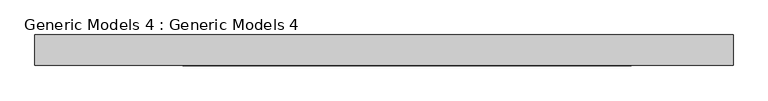
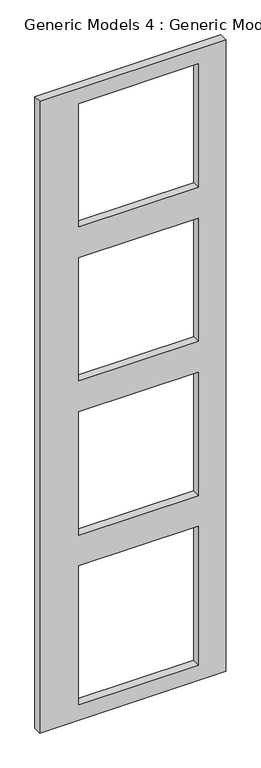
"""IFC4 building model written with IfcOpenShell, lengths in millimetres: proxy geometry, Generic Models 4 : Generic Models 4."""

from ifc_helpers import new_model, si_unit, frame, origin, place, context, project, spatial, polyline, outline, extrude, source, transform, mapped, element, save


def generic_models_4_generic_models_4_3a94e551(model_context):
    return source(origin(), model_context, "Body", "SweptSolid", [
        extrude(outline(polyline([(12192.0, 5154.8072267), (12192.0, 1674.8824202), (-304.8, 1674.8824202), (-304.8, 5154.8072267), (12192.0, 5154.8072267)]), holes=[polyline([(11887.2, 4646.6824202), (9448.8, 4646.6824202), (9448.8, 2411.4824202), (11887.2, 2411.4824202), (11887.2, 4646.6824202)]), polyline([(8839.2, 4646.6824202), (6400.8, 4646.6824202), (6400.8, 2411.4824202), (8839.2, 2411.4824202), (8839.2, 4646.6824202)]), polyline([(5791.2, 4646.6824202), (3352.8, 4646.6824202), (3352.8, 2411.4824202), (5791.2, 2411.4824202), (5791.2, 4646.6824202)]), polyline([(2743.2, 4646.6824202), (0.0, 4646.6824202), (0.0, 2411.4824202), (2743.2, 2411.4824202), (2743.2, 4646.6824202)])]), frame((0.0, -14729.2402089, 0.0), z_axis=(0.0, 1.0, 0.0), x_axis=(0.0, 0.0, 1.0)), (0.0, 0.0, 1.0), 152.4),
    ])


if __name__ == "__main__":
    model = new_model("IFC4")
    model_context = context("Model", 3, world=origin())
    ifc_project = project(units=[si_unit("LENGTHUNIT", "METRE", prefix="MILLI")], contexts=[model_context])
    site = spatial("IfcSite", under=ifc_project)
    building = spatial("IfcBuilding", under=site)
    placement = place(None, origin())
    generic_models_4_generic_models_4_shape = generic_models_4_generic_models_4_3a94e551(model_context)
    element("IfcBuildingElementProxy", 1, Name="Generic Models 4 : Generic Models 4", ObjectType="Generic Models 4 : Generic Models 4", at=placement, inside=building, context=model_context, shape_type="MappedRepresentation", body=[
        mapped(generic_models_4_generic_models_4_shape, transform((0.0, 0.0, 0.0), x_axis=(1.0, 0.0, 0.0), y_axis=(0.0, 1.0, 0.0), z_axis=(0.0, 0.0, 1.0))),
    ])
    save(model, "model.ifc")

# Revit data of these elements
# Element 1 (IfcBuildingElementProxy, "Generic Models 4 : Generic Models 4")
#   Materials on its faces: "black accent wall"
# Materials
#   "black accent wall": class "Generic", colour RGB 120 120 120, transparency 0, Cost = 0
